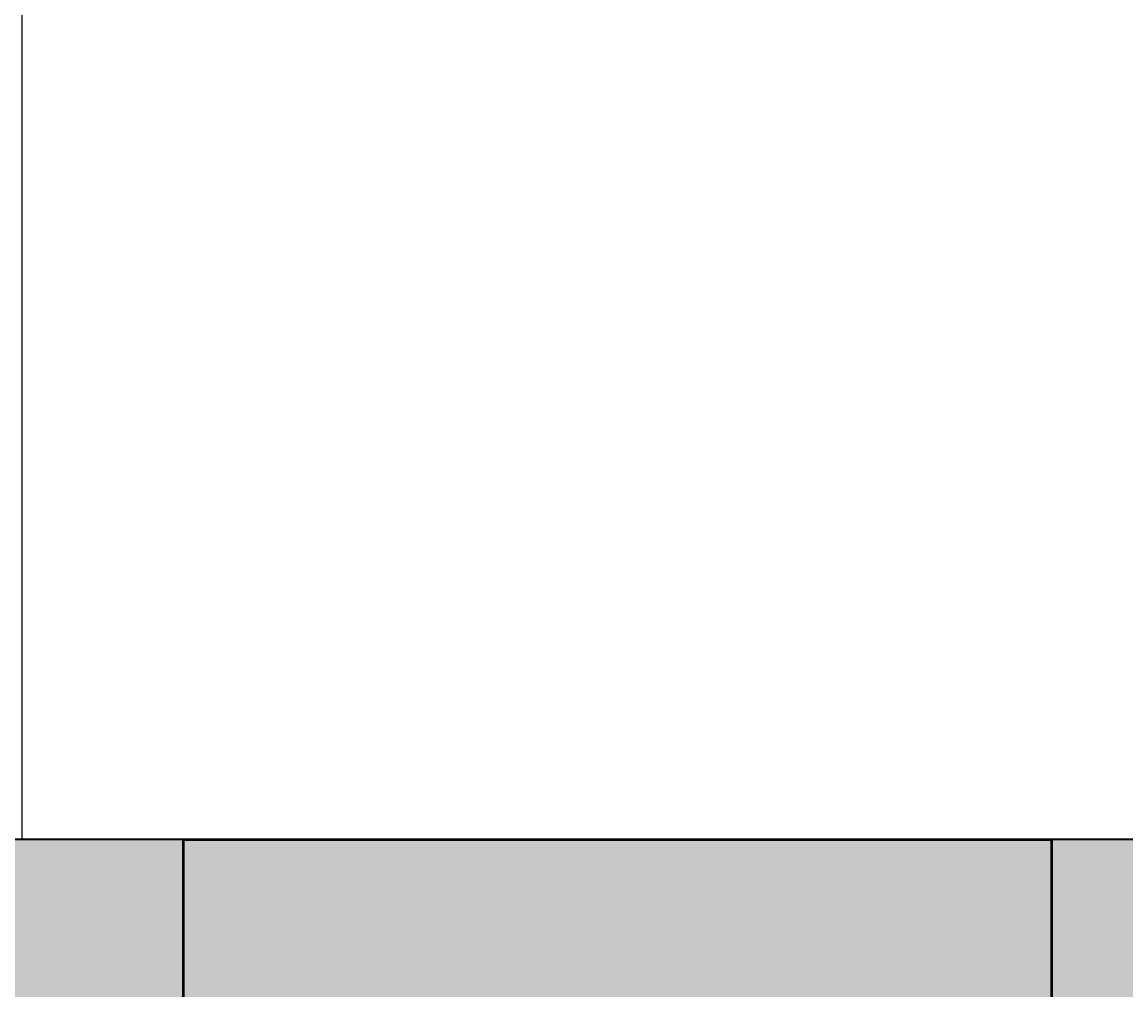
# Model space of a CAD drawing. Units: inches. Extents: x 1998 to 2588, y 1139 to 1977.
# Tile 113 of 134: x 2498 to 2524, y 1477 to 1500. Entities that reach past the tile are written whole.
import ezdxf

# ---------------------------------------------------------------- set-up
doc = ezdxf.new("R2010")
doc.units = ezdxf.units.IN
for name, color, linetype, lineweight in [('A-ANNO-DIMS', 2, 'Continuous', 18), ('A-COLS-PATT', 250, 'Continuous', 13), ('A-FLOR-STRS', 7, 'Continuous', 25), ('A-WALL-PATT', 252, 'Continuous', 13), ('COLUMN', 10, 'Continuous', 50), ('WALL', 200, 'Continuous', 35)]:
    doc.layers.add(name, color=color, linetype=linetype, lineweight=lineweight)
doc.styles.get("Standard").update_dxf_attribs({"font": 'arial.ttf'})
doc.dimstyles.get("Standard").update_dxf_attribs({"dimtxt": 0.18, "dimasz": 0.18, "dimexe": 0.18, "dimexo": 0.0625, "dimgap": 0.09, "dimtad": 0, "dimtih": 1, "dimtoh": 1, "dimdec": 4, "dimzin": 0, "dimdsep": 46, "dimtxsty": 'Standard', "dimcen": 0.09, "dimadec": 0, "dimazin": 0, "dimtfac": 1, "dimtdec": 4, "dimtofl": 0, "dimtmove": 0, "dimatfit": 3, "dimfxl": 1, "dimtolj": 1, "dimtzin": 0, "dimarcsym": 0})

# ---------------------------------------------------------------- blocks, each defined once
blk = doc.blocks.new('*D24')
at = {"layer": 'A-ANNO-DIMS', "color": 0, "lineweight": -2, "transparency": 16777216}
for p, q in [((2398.535, 1911.232), (2588.309, 1911.232)), ((2588.129, 1911.052), (2588.129, 1570.164)), ((2588.129, 1228.912), (2588.129, 1569.8)), ((2527.535, 1228.732), (2588.309, 1228.732))]:
    blk.add_line(p, q, dxfattribs=at)
at = {"layer": 'A-ANNO-DIMS', "color": 0, "transparency": 16777216}
for points in [[(2588.099, 1911.052), (2588.159, 1911.052), (2588.129, 1911.232)], [(2588.099, 1228.912), (2588.159, 1228.912), (2588.129, 1228.732)]]:
    blk.add_solid(points, dxfattribs=at)
at = {"layer": 'Defpoints', "color": 0, "transparency": 16777216}
for p in [(2398.473, 1911.232), (2588.129, 1911.232), (2527.473, 1228.732)]:
    blk.add_point(p, dxfattribs=at)
at = {"layer": 'A-ANNO-DIMS', "color": 0, "transparency": 16777216, "insert": (2588.129, 1569.982), "char_height": 0.18, "attachment_point": 5}
blk.add_mtext('\\A1;682.5', dxfattribs=at)

msp = doc.modelspace()

# ---------------------------------------------------------------- hatches: boundary and pattern name
at = {"layer": 'A-COLS-PATT'}
h = msp.add_hatch(color=256, dxfattribs=at)
h.dxf.hatch_style = 1
h.paths.add_polyline_path([(2099.4125, 1888.7324), (2087.9729, 1888.7324), (2087.9729, 1868.3278), (2099.4125, 1868.3278)])
h.paths.add_polyline_path([(2234.4125, 1888.7324), (2222.9729, 1888.7324), (2222.9729, 1868.3278), (2234.4125, 1868.3278)])
h.paths.add_polyline_path([(2341.4729, 1886.637), (2330.0332, 1886.637), (2330.0332, 1866.2324), (2341.4729, 1866.2324)])
h.paths.add_polyline_path([(2507.8006, 1882.7324), (2487.396, 1882.7324), (2487.396, 1871.2927), (2507.8006, 1871.2927)])
h.paths.add_polyline_path([(2510.9729, 1766.672), (2490.5682, 1766.672), (2490.5682, 1755.2324), (2510.9729, 1755.2324)])
h.paths.add_polyline_path([(2345.9729, 1759.7324), (2334.5332, 1759.7324), (2334.5332, 1739.3278), (2345.9729, 1739.3278)])
h.paths.add_polyline_path([(2234.4125, 1774.3318), (2222.9729, 1774.3318), (2222.9729, 1753.9272), (2234.4125, 1753.9272)])
h.paths.add_polyline_path([(2099.4125, 1775.637), (2087.9729, 1775.637), (2087.9729, 1755.2324), (2099.4125, 1755.2324)])
h.paths.add_polyline_path([(2098.0956, 1593.7241), (2077.691, 1593.7241), (2077.691, 1582.2845), (2098.0956, 1582.2845)])
h.paths.add_polyline_path([(2227.4729, 1604.637), (2216.0332, 1604.637), (2216.0332, 1584.2324), (2227.4729, 1584.2324)])
h.paths.add_polyline_path([(2345.9729, 1647.5211), (2334.5332, 1647.5211), (2334.5332, 1627.1165), (2345.9729, 1627.1165)])
h.paths.add_polyline_path([(2522.3775, 1641.2324), (2501.9729, 1641.2324), (2501.9729, 1629.7927), (2522.3775, 1629.7927)])
h.paths.add_polyline_path([(2522.3775, 1480.7324), (2501.9729, 1480.7324), (2501.9729, 1469.2927), (2522.3775, 1469.2927)])
h.paths.add_polyline_path([(2345.9729, 1488.5616), (2334.5332, 1488.5616), (2334.5332, 1468.1569), (2345.9729, 1468.1569)])
h.paths.add_polyline_path([(2234.4125, 1486.137), (2227.4729, 1486.137), (2227.4729, 1465.7324), (2234.4125, 1465.7324)])
h.paths.add_polyline_path([(2227.4729, 1486.137), (2222.9729, 1486.137), (2222.9729, 1465.7324), (2227.4729, 1465.7324)])
h.paths.add_polyline_path([(2108.3775, 1470.2324), (2087.9729, 1470.2324), (2087.9729, 1458.7927), (2108.3775, 1458.7927)])
h.paths.add_polyline_path([(2096.9729, 1365.5012), (2087.9729, 1365.5012), (2087.9729, 1345.0966), (2096.9729, 1345.0966)])
h.paths.add_polyline_path([(2087.9729, 1365.5012), (2085.5332, 1365.5012), (2085.5332, 1345.0966), (2087.9729, 1345.0966)])
h.paths.add_polyline_path([(2234.4125, 1285.137), (2222.9729, 1285.137), (2222.9729, 1264.7324), (2234.4125, 1264.7324)])
h.paths.add_polyline_path([(2345.9729, 1285.137), (2334.5332, 1285.137), (2334.5332, 1264.7324), (2345.9729, 1264.7324)])
h.paths.add_polyline_path([(2503.1458, 1240.172), (2482.7412, 1240.172), (2482.7412, 1228.7324), (2503.1458, 1228.7324)])
h.paths.add_polyline_path([(2510.9729, 1369.172), (2490.5682, 1369.172), (2490.5682, 1357.7324), (2510.9729, 1357.7324)])
at = {"layer": 'A-WALL-PATT'}
h = msp.add_hatch(color=256, dxfattribs=at)
h.dxf.hatch_style = 1
h.paths.add_polyline_path([(2527.4729, 1362.2324), (2510.9729, 1362.2324), (2510.9729, 1357.7324), (2518.4729, 1357.7324), (2518.4729, 1237.7324), (2503.1458, 1237.7324), (2503.1458, 1228.7324), (2527.4729, 1228.7324)])
h.paths.add_polyline_path([(2490.5682, 1362.2324), (2398.4729, 1362.2324), (2398.4729, 1357.7324), (2490.5682, 1357.7324)])
h.paths.add_polyline_path([(2224.9729, 1264.7324), (2222.9729, 1264.7324), (2222.9729, 1232.4125), (2341.4729, 1232.4125), (2341.4729, 1234.4125), (2224.9729, 1234.4125)])
h.paths.add_polyline_path([(2334.5332, 1273.7324), (2264.7638, 1273.7324), (2264.7638, 1269.5611, -0.043659), (2264.3413, 1264.7324), (2334.5332, 1264.7324)])
h.paths.add_polyline_path([(2236.9551, 1273.7324), (2234.4125, 1273.7324), (2234.4125, 1264.7324), (2236.9551, 1264.7324), (2236.9551, 1269.5611)])
h.paths.add_polyline_path([(2222.9729, 1293.2324), (2096.9729, 1293.2324), (2096.9729, 1345.0966), (2087.9729, 1345.0966), (2087.9729, 1284.2324), (2222.9729, 1284.2324), (2222.9729, 1285.137)])
h.paths.add_polyline_path([(2096.9729, 1458.7927), (2087.9729, 1458.7927), (2087.9729, 1417.7324), (2087.9729, 1413.2324), (2096.9729, 1413.2324), (2096.9729, 1417.7324)])
h.paths.add_polyline_path([(2096.9729, 1413.2324), (2087.9729, 1413.2324), (2087.9729, 1365.5012), (2096.9729, 1365.5012), (2096.9729, 1369.3358)])
h.paths.add_polyline_path([(2186.2943, 1417.7324), (2138.6074, 1417.7324), (2096.9729, 1417.7324), (2096.9729, 1413.2324), (2138.6074, 1413.2324), (2186.2943, 1413.2324)])
h.paths.add_polyline_path([(2181.4729, 1465.7324), (2176.9729, 1465.7324), (2176.9729, 1451.6434), (2181.4729, 1451.6434)])
h.paths.add_polyline_path([(2181.4729, 1422.1664), (2176.9729, 1422.1664), (2176.9729, 1417.7324), (2181.4729, 1417.7324)])
h.paths.add_polyline_path([(2063.9729, 1465.7324), (2087.9729, 1465.7324), (2087.9729, 1470.2324), (2059.4729, 1470.2324), (2059.4729, 1413.2324), (2087.9729, 1413.2324), (2087.9729, 1417.7324), (2063.9729, 1417.7324)])
h.paths.add_polyline_path([(2181.4729, 1755.2324), (2176.9729, 1755.2324), (2176.9729, 1748.6798), (2177.0513, 1748.6798), (2181.4729, 1748.6798)])
h.paths.add_polyline_path([(2227.4729, 1707.2324), (2220.4647, 1707.2324), (2220.4647, 1702.7324), (2222.9729, 1702.7324), (2222.9729, 1604.637), (2227.4729, 1604.637)])
h.paths.add_polyline_path([(2114.9729, 1702.7324), (2105.9729, 1702.7324), (2105.9729, 1628.4781, -0.0318759), (2110.1012, 1628.7416), (2114.9729, 1628.7416)])
h.paths.add_polyline_path([(2345.9729, 1739.3278), (2341.4729, 1739.3278), (2341.4729, 1647.5211), (2345.9729, 1647.5211)])
h.paths.add_polyline_path([(2350.6273, 1641.2324), (2345.9729, 1641.2324), (2345.9729, 1636.7324), (2350.6273, 1636.7324), (2350.6273, 1639.8729)])
h.paths.add_polyline_path([(2501.9729, 1641.2324), (2407.9729, 1641.2324), (2392.5005, 1641.2324), (2392.5005, 1639.8729), (2392.5005, 1636.7324), (2501.9729, 1636.7324)])
h.paths.add_polyline_path([(2510.9729, 1755.2324), (2501.9729, 1755.2324), (2501.9729, 1641.2324), (2510.9729, 1641.2324)])
h.paths.add_polyline_path([(2549.1786, 1641.2324), (2522.3775, 1641.2324), (2522.3775, 1636.7324), (2540.1786, 1636.7324), (2540.1786, 1480.7324), (2522.3775, 1480.7324), (2522.3775, 1476.2324), (2549.1786, 1476.2324)])
h.paths.add_polyline_path([(2498.1786, 1594.7324), (2407.9729, 1594.7324), (2407.9729, 1585.7324), (2416.9729, 1585.7324), (2489.1786, 1585.7324), (2489.1786, 1531.7324), (2416.9729, 1531.7324), (2407.9729, 1531.7324), (2407.9729, 1522.7324), (2498.1786, 1522.7324)])
h.paths.add_polyline_path([(2351.6437, 1480.7324), (2345.9729, 1480.7324), (2345.9729, 1476.2324), (2351.6437, 1476.2324), (2351.6437, 1477.5919)])
h.paths.add_polyline_path([(2501.9729, 1480.7324), (2498.1786, 1480.7324), (2407.9729, 1480.7324), (2393.5168, 1480.7324), (2393.5168, 1477.5919), (2393.5168, 1476.2324), (2501.9729, 1476.2324)])

# ---------------------------------------------------------------- linework, layer by layer
at = {"layer": 'A-FLOR-STRS'}
for p, q in [((2498.1786, 1480.7324), (2498.1786, 1636.7324)), ((2498.1786, 1480.7324), (2498.1786, 1522.7324)), ((2540.1786, 1480.7324), (2498.1786, 1480.7324))]:
    msp.add_line(p, q, dxfattribs=at)
at = {"layer": 'COLUMN'}
msp.add_lwpolyline([(2522.3775, 1480.7324), (2522.3775, 1469.2927), (2501.9729, 1469.2927), (2501.9729, 1480.7324)], close=True, dxfattribs=at)
at = {"layer": 'WALL'}
msp.add_line((2540.1786, 1480.7324), (2407.9729, 1480.7324), dxfattribs=at)

# ---------------------------------------------------------------- dimensions: what is measured, and where the dimension line sits
at = {"layer": 'A-ANNO-DIMS'}
dim = msp.add_linear_dim(base=(2588.1286, 1911.2324), p1=(2527.4729, 1228.7324), p2=(2398.4729, 1911.2324), angle=90, dimstyle='Standard', override={"dimdec": 1, "dimlfac": 1, "dimrnd": 0, "dimzin": 0, "dimdsep": 46, "dimlunit": 2}, dxfattribs=at)
dim.commit()
dim.dimension.update_dxf_attribs({"geometry": '*D24', "text_midpoint": (2588.1286, 1569.9824)})

doc.saveas('drawing.dxf')
